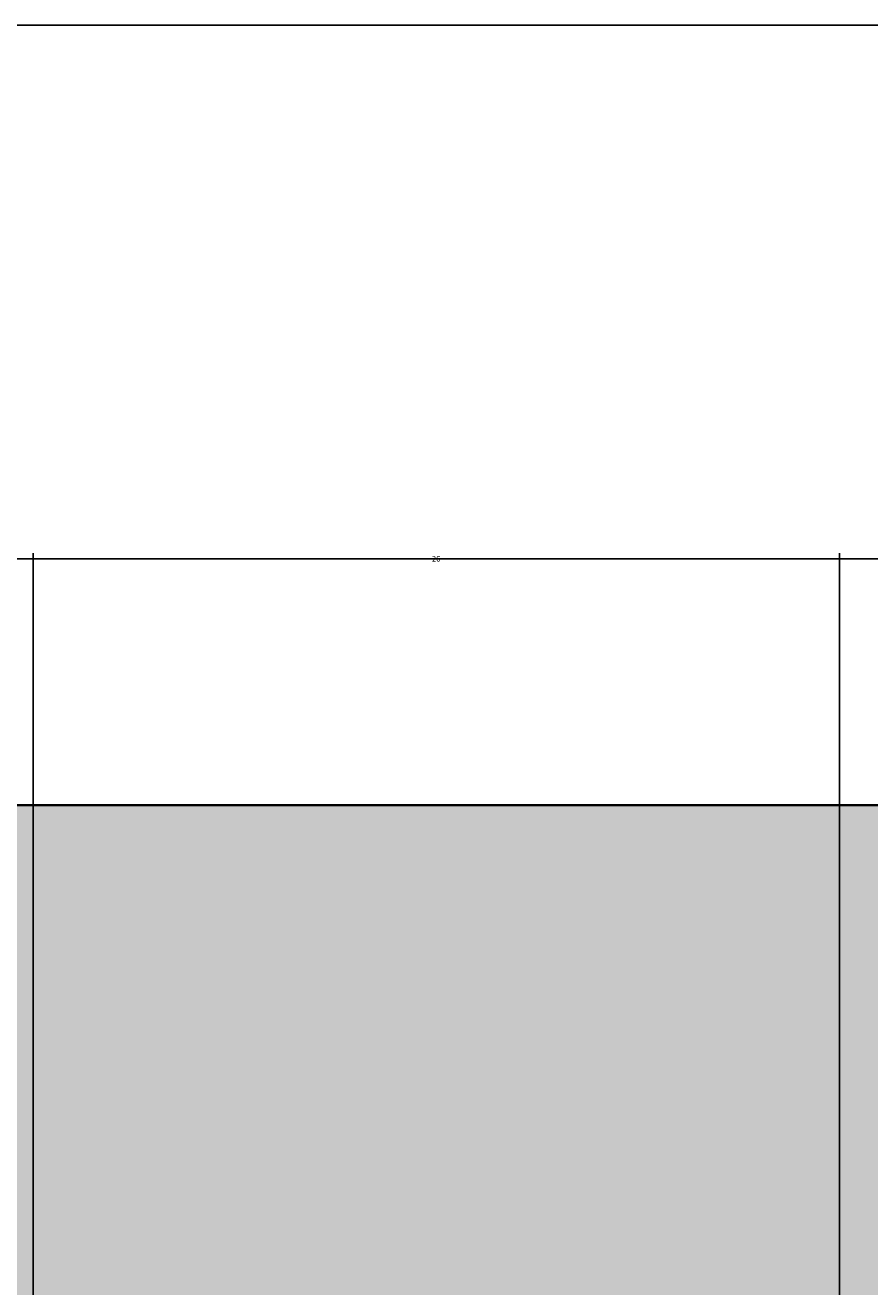
# Model space of a CAD drawing. Units: inches. Extents: x 4508 to 4723, y 847 to 1020.
# Tile 29 of 32: x 4631 to 4658, y 979 to 1020. Entities that reach past the tile are written whole.
import ezdxf

# ---------------------------------------------------------------- set-up
doc = ezdxf.new("R2010")
doc.units = ezdxf.units.IN
for name, color, linetype, lineweight in [('A-ANNO-DIMS', 2, 'Continuous', 18), ('A-ANNO-TTLB', 7, 'Continuous', 25), ('A-WALL', 7, 'Continuous', 35), ('A-WALL-PATT', 254, 'Continuous', 13)]:
    doc.layers.add(name, color=color, linetype=linetype, lineweight=lineweight)
doc.styles.get("Standard").update_dxf_attribs({"font": 'arial.ttf'})
doc.dimstyles.get("Standard").update_dxf_attribs({"dimtxt": 0.18, "dimasz": 0.18, "dimexe": 0.18, "dimexo": 0.0625, "dimgap": 0.09, "dimtad": 0, "dimtih": 1, "dimtoh": 1, "dimdec": 4, "dimzin": 0, "dimdsep": 46, "dimtxsty": 'Standard', "dimcen": 0.09, "dimadec": 0, "dimazin": 0, "dimtfac": 1, "dimtdec": 4, "dimtofl": 0, "dimtmove": 0, "dimatfit": 3, "dimfxl": 1, "dimtolj": 1, "dimtzin": 0, "dimarcsym": 0})

# ---------------------------------------------------------------- blocks, each defined once
blk = doc.blocks.new('*D7')
at = {"layer": 'A-ANNO-DIMS', "color": 0, "lineweight": -2, "transparency": 16777216}
for p, q in [((4588.994, 994.809), (4588.994, 1002.877)), ((4589.174, 1002.697), (4625.189, 1002.697)), ((4661.991, 1002.697), (4625.975, 1002.697)), ((4662.171, 957.665), (4662.171, 1002.877))]:
    blk.add_line(p, q, dxfattribs=at)
at = {"layer": 'A-ANNO-DIMS', "color": 0, "lineweight": 9, "transparency": 16777216}
for points in [[(4589.174, 1002.727), (4589.174, 1002.667), (4588.994, 1002.697)], [(4661.991, 1002.727), (4661.991, 1002.667), (4662.171, 1002.697)]]:
    blk.add_solid(points, dxfattribs=at)
at = {"layer": 'Defpoints', "color": 0, "lineweight": 9, "transparency": 16777216}
for p in [(4662.171, 1002.697), (4588.994, 994.747), (4662.171, 957.602)]:
    blk.add_point(p, dxfattribs=at)
at = {"layer": 'A-ANNO-DIMS', "color": 0, "transparency": 16777216, "insert": (4625.582, 1002.697), "char_height": 0.18, "attachment_point": 5}
blk.add_mtext('\\A1;73.18', dxfattribs=at)
blk = doc.blocks.new('*D31')
at = {"layer": 'A-ANNO-DIMS', "color": 0, "lineweight": -2, "transparency": 16777216}
for p, q in [((4630.994, 903.809), (4630.994, 1002.877)), ((4631.174, 1002.697), (4643.773, 1002.697)), ((4656.814, 1002.697), (4644.214, 1002.697)), ((4656.994, 903.809), (4656.994, 1002.877))]:
    blk.add_line(p, q, dxfattribs=at)
at = {"layer": 'A-ANNO-DIMS', "color": 0, "lineweight": 9, "transparency": 16777216}
for points in [[(4631.174, 1002.727), (4631.174, 1002.667), (4630.994, 1002.697)], [(4656.814, 1002.727), (4656.814, 1002.667), (4656.994, 1002.697)]]:
    blk.add_solid(points, dxfattribs=at)
at = {"layer": 'Defpoints', "color": 0, "lineweight": 9, "transparency": 16777216}
for p in [(4656.994, 1002.697), (4630.994, 903.747), (4656.994, 903.747)]:
    blk.add_point(p, dxfattribs=at)
at = {"layer": 'A-ANNO-DIMS', "color": 0, "transparency": 16777216, "insert": (4643.994, 1002.697), "char_height": 0.18, "attachment_point": 5}
blk.add_mtext('\\A1;26', dxfattribs=at)

msp = doc.modelspace()

# ---------------------------------------------------------------- hatches: boundary and pattern name
at = {"layer": 'A-WALL-PATT', "transparency": 33554508}
h = msp.add_hatch(color=256, dxfattribs=at)
h.dxf.hatch_style = 1
h.paths.add_polyline_path([(4661.6706, 954.043, -0.3739004), (4658.5765, 957.6021, -1), (4665.7646, 957.6021, -0.3739004), (4662.6706, 954.043), (4662.6706, 944.4021, -0.2114781), (4670.3062, 945.0869), (4670.3062, 968.0592, -0.4632086), (4663.3246, 973.9783, -0.4632086), (4670.3062, 979.8975), (4670.3062, 994.7469), (4588.9938, 994.7469), (4588.9938, 904.7469), (4657.9938, 904.7469), (4657.9938, 886.7469), (4549.9938, 886.7469), (4549.9938, 878.7469), (4693.9938, 878.7469), (4693.9938, 994.7469), (4671.8062, 994.7469), (4671.8062, 979.4411, -0.2941682), (4675.3246, 973.9783, -0.2941682), (4671.8062, 968.5156), (4671.8062, 944.4278, -0.2741114), (4676.7298, 936.1217, -0.2741114), (4671.8062, 927.8155), (4671.8062, 907.6998, -0.3779645), (4677.0562, 901.7469, -0.3779645), (4671.8062, 895.7939), (4671.8062, 883.7469), (4670.3062, 883.7469), (4670.3062, 895.7939, -0.3779645), (4665.0562, 901.7469, -0.3779645), (4670.3062, 907.6998), (4670.3062, 927.1564, -0.2114781), (4662.6706, 927.8412), (4662.6706, 918.2003, -0.3739004), (4665.7646, 914.6412, -1), (4658.5765, 914.6412, -0.3739004), (4661.6706, 918.2003), (4661.6706, 928.4807, -0.2391825), (4657.7936, 936.1217, -0.2391825), (4661.6706, 943.7626)])

# ---------------------------------------------------------------- linework, layer by layer
at = {"layer": 'A-ANNO-TTLB'}
msp.add_lwpolyline([(4508.3867, 1019.9118), (4722.9774, 1019.9118), (4722.9774, 846.9535), (4508.3867, 846.9535)], close=True, dxfattribs=at)
at = {"layer": 'A-WALL'}
msp.add_line((4540.9938, 994.7469), (4693.9938, 994.7469), dxfattribs=at)

# ---------------------------------------------------------------- dimensions: what is measured, and where the dimension line sits
at = {"layer": 'A-ANNO-DIMS'}
for base, p1, p2, override, picture, middle in [((4662.1706, 1002.6969), (4588.9938, 994.7469), (4662.1706, 957.6021), {"dimdec": 2, "dimlfac": 1, "dimrnd": 0, "dimzin": 0, "dimdsep": 46, "dimlunit": 2}, '*D7', (4625.5822, 1002.6969)), ((4656.9938, 1002.6969), (4630.9938, 903.7469), (4656.9938, 903.7469), {"dimdec": 0, "dimlfac": 1, "dimrnd": 0, "dimzin": 0, "dimdsep": 46, "dimlunit": 2}, '*D31', (4643.9938, 1002.6969))]:
    dim = msp.add_linear_dim(base=base, p1=p1, p2=p2, dimstyle='Standard', override=override, dxfattribs=at)
    dim.commit()
    dim.dimension.update_dxf_attribs({"geometry": picture, "text_midpoint": middle})

doc.saveas('drawing.dxf')
